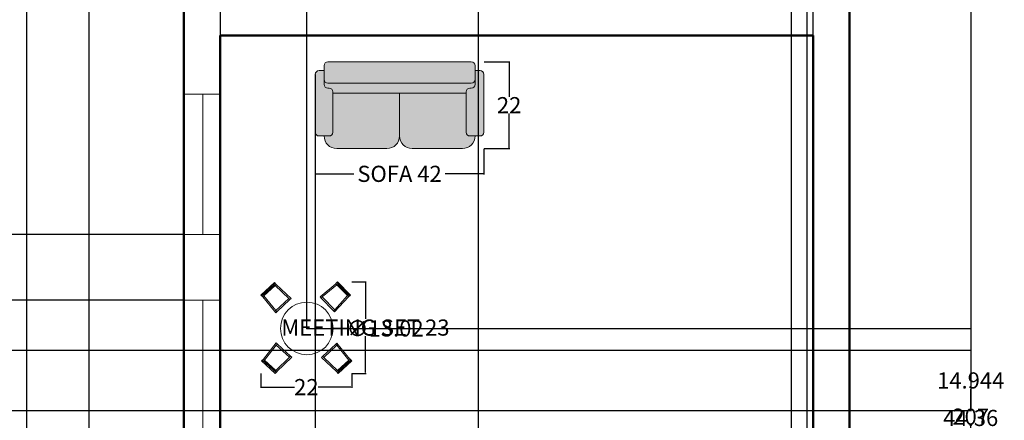
# Model space of a CAD drawing. Units: inches. Extents: x 1454 to 2136, y 626 to 1213.
# Tile 22 of 23: x 1887 to 2131, y 806 to 905. Entities that reach past the tile are written whole.
import ezdxf

# ---------------------------------------------------------------- set-up
doc = ezdxf.new("R2010")
doc.units = ezdxf.units.IN
doc.header["$MEASUREMENT"] = 0
for name, color, linetype, lineweight in [('A-ANNO-DIMS', 2, 'Continuous', 18), ('A-FURN-PATT', 252, 'Continuous', 13), ('A-GLAZ', 4, 'Continuous', 18), ('A-WALL', 7, 'Continuous', 50), ('conference', 41, 'Continuous', 18), ('sofa', 4, 'Continuous', 18)]:
    doc.layers.add(name, color=color, linetype=linetype, lineweight=lineweight)
doc.styles.get("Standard").update_dxf_attribs({"font": 'arial.ttf'})
doc.dimstyles.get("Standard").update_dxf_attribs({"dimtxt": 4, "dimasz": 0.18, "dimexe": 0.18, "dimexo": 0.0625, "dimgap": 0.09, "dimtad": 0, "dimtih": 1, "dimtoh": 1, "dimdec": 0, "dimrnd": 6, "dimzin": 0, "dimdsep": 46, "dimlunit": 3, "dimtxsty": 'Standard', "dimcen": 0.09, "dimadec": 0, "dimazin": 0, "dimtfac": 1, "dimtdec": 0, "dimtofl": 0, "dimtmove": 0, "dimatfit": 3, "dimfxl": 1, "dimtolj": 1, "dimtzin": 0, "dimarcsym": 0})

# ---------------------------------------------------------------- blocks, each defined once
blk = doc.blocks.new('A$C02A636C4')
for p, q in [((0.0679, 0.6401), (0.0679, 0.6013)), ((1.2026, 0.6692), (0.097, 0.6692)), ((1.2317, 0.6401), (1.2317, 0.6013)), ((0, 0.5722), (0, 0.1261)), ((0.0679, 0.6013), (0.0291, 0.6013)), ((0.0679, 0.5334), (0.0679, 0.6013)), ((0.0679, 0.4946), (0.0679, 0.5431)), ((1.2317, 0.6013), (1.2705, 0.6013)), ((1.2317, 0.5334), (1.2317, 0.6013)), ((1.2317, 0.4946), (1.2317, 0.5431)), ((1.2996, 0.5722), (1.2996, 0.1261)), ((1.2026, 0.5043), (0.097, 0.5043)), ((0.1067, 0.4655), (0.097, 0.4655)), ((1.1929, 0.4655), (1.2026, 0.4655)), ((0.1358, 0.1261), (0.1358, 0.4364)), ((1.1638, 0.4267), (0.1358, 0.4267)), ((0.6498, 0.097), (0.6498, 0.4267)), ((1.1638, 0.1261), (1.1638, 0.4364)), ((0.0291, 0.097), (0.1067, 0.097)), ((1.2705, 0.097), (1.1929, 0.097)), ((0.1649, 0), (0.5528, 0)), ((0.7468, 0), (1.1347, 0))]:
    blk.add_line(p, q)
for centre, radius, start, end in [((0.097, 0.6401), 0.0291, 90, 180), ((1.2026, 0.6401), 0.0291, 0, 90), ((0.0291, 0.5722), 0.0291, 90, 180), ((0.097, 0.5334), 0.0291, 180, 270), ((1.2026, 0.5334), 0.0291, 270, 0), ((1.2705, 0.5722), 0.0291, 0, 90), ((0.097, 0.4946), 0.0291, 180, 270), ((0.1067, 0.4364), 0.0291, 0, 90), ((1.1929, 0.4364), 0.0291, 90, 180), ((1.2026, 0.4946), 0.0291, 270, 0), ((0.0291, 0.1261), 0.0291, 180, 270), ((0.1649, 0.097), 0.097, 180, 270), ((0.1067, 0.1261), 0.0291, 270, 0), ((0.5528, 0.097), 0.097, 270, 0), ((0.7468, 0.097), 0.097, 180, 270), ((1.1347, 0.097), 0.097, 270, 0), ((1.1929, 0.1261), 0.0291, 180, 270), ((1.2705, 0.1261), 0.0291, 270, 0)]:
    blk.add_arc(centre, radius, start, end)
blk = doc.blocks.new('ОГ018 на4персон столR500')
for p, q in [((-616, 874), (-872, 635)), ((-601, 858), (-857, 620)), ((-604, 817), (-816, 620)), ((-699, 740), (-713, 755)), ((-705, 761), (-691, 747)), ((-666, 787), (-700, 756)), ((-658, 778), (-672, 793)), ((-664, 800), (-651, 785)), ((-625, 825), (-659, 794)), ((-651, 785), (-658, 778)), ((-612, 811), (-631, 831)), ((-582, 838), (-616, 874)), ((-582, 838), (-604, 817)), ((-340, 571), (-604, 817)), ((-298, 570), (-584, 837)), ((252, 600), (551, 852)), ((294, 600), (571, 832)), ((550, 854), (585, 888)), ((550, 854), (571, 832)), ((570, 873), (813, 621)), ((571, 832), (772, 624)), ((578, 825), (598, 844)), ((585, 888), (829, 636)), ((592, 839), (624, 806)), ((630, 811), (615, 797)), ((615, 797), (622, 790)), ((622, 790), (637, 804)), ((631, 798), (663, 765)), ((669, 771), (654, 757)), ((654, 757), (661, 750)), ((661, 750), (676, 764)), ((670, 758), (702, 725)), ((-838, 599), (-872, 635)), ((-816, 620), (-838, 599)), ((-837, 600), (-591, 297)), ((-809, 626), (-828, 647)), ((-789, 672), (-823, 641)), ((-816, 620), (-589, 339)), ((-781, 663), (-794, 678)), ((-787, 685), (-773, 670)), ((-748, 711), (-782, 679)), ((-773, 670), (-781, 663)), ((-740, 702), (-754, 716)), ((-746, 723), (-732, 708)), ((-707, 749), (-741, 717)), ((-732, 708), (-740, 702)), ((-691, 747), (-699, 740)), ((-589, 339), (-340, 571)), ((-341, 571), (-320, 549)), ((-340, 571), (-320, 549)), ((-320, 549), (-298, 570)), ((-320, 549), (-298, 570)), ((273, 579), (252, 601)), ((273, 579), (252, 600)), ((294, 600), (273, 579)), ((295, 600), (273, 579)), ((509, 334), (273, 579)), ((531, 355), (294, 600)), ((792, 603), (530, 313)), ((772, 624), (531, 355)), ((707, 731), (693, 717)), ((693, 717), (700, 709)), ((700, 709), (714, 723)), ((709, 718), (741, 685)), ((746, 690), (732, 676)), ((732, 676), (739, 669)), ((739, 669), (753, 683)), ((748, 678), (780, 645)), ((765, 631), (785, 650)), ((772, 624), (793, 602)), ((793, 602), (829, 636)), ((-569, 317), (-320, 549)), ((-591, 297), (-569, 317)), ((-591, 297), (-569, 317)), ((-569, 317), (-589, 339)), ((509, 334), (531, 355)), ((530, 313), (509, 334)), ((530, 313), (509, 334)), ((-824, -584), (-582, -277)), ((-803, -603), (-580, -320)), ((-582, -277), (-559, -297)), ((-582, -277), (-559, -297)), ((-559, -297), (-580, -320)), ((-580, -320), (-328, -548)), ((-559, -297), (-308, -526)), ((551, -299), (303, -530)), ((572, -321), (323, -552)), ((573, -278), (551, -299)), ((573, -278), (551, -299)), ((551, -299), (572, -321)), ((799, -601), (572, -321)), ((820, -582), (573, -278)), ((-328, -548), (-588, -798)), ((-285, -546), (-567, -817)), ((-328, -548), (-308, -526)), ((-328, -548), (-308, -526)), ((-308, -526), (-285, -546)), ((-308, -526), (-285, -546)), ((303, -530), (281, -551)), ((303, -530), (281, -551)), ((281, -551), (566, -818)), ((323, -552), (303, -530)), ((323, -552), (303, -530)), ((323, -552), (587, -799)), ((-825, -583), (-859, -619)), ((-599, -855), (-859, -619)), ((-585, -839), (-844, -603)), ((-803, -603), (-825, -583)), ((-796, -610), (-814, -630)), ((-775, -655), (-809, -624)), ((-588, -798), (-803, -603)), ((-767, -646), (-780, -661)), ((-773, -668), (-759, -653)), ((-734, -693), (-768, -662)), ((-759, -653), (-767, -646)), ((-725, -684), (-739, -699)), ((-732, -706), (-718, -691)), ((-692, -731), (-726, -700)), ((-718, -691), (-725, -684)), ((-684, -722), (-697, -736)), ((-690, -743), (-677, -728)), ((-651, -768), (-685, -737)), ((-677, -728), (-684, -722)), ((584, -839), (840, -601)), ((587, -799), (799, -601)), ((599, -855), (855, -617)), ((649, -768), (682, -737)), ((674, -728), (681, -721)), ((688, -743), (674, -728)), ((681, -721), (695, -736)), ((690, -730), (723, -699)), ((715, -690), (722, -683)), ((729, -704), (715, -690)), ((722, -683), (736, -698)), ((731, -692), (764, -661)), ((756, -652), (763, -645)), ((770, -666), (756, -652)), ((763, -645), (777, -659)), ((772, -654), (805, -622)), ((792, -608), (811, -628)), ((799, -601), (821, -580)), ((821, -580), (855, -617)), ((-642, -759), (-656, -774)), ((-649, -781), (-635, -766)), ((-609, -806), (-643, -775)), ((-635, -766), (-642, -759)), ((-596, -791), (-615, -812)), ((-566, -818), (-599, -855)), ((-566, -818), (-588, -798)), ((565, -819), (587, -799)), ((565, -819), (599, -855)), ((594, -792), (613, -812)), ((608, -806), (641, -775)), ((633, -766), (640, -759)), ((647, -781), (633, -766)), ((640, -759), (654, -774))]:
    blk.add_line(p, q)
blk.add_circle((0, 0), 500)
for p in [(-589, 339), (531, 355), (-580, -320), (572, -321)]:
    blk.add_point(p)
blk = doc.blocks.new('WIN-34_84')
blk.add_line((34.84, 4.31), (0, 4.31))
blk.add_lwpolyline([(34.84, 0), (0, 0), (0, 9), (34.84, 9)], close=True)
blk = doc.blocks.new('*D21')
at = {"layer": 'A-ANNO-DIMS', "color": 0, "lineweight": -2, "transparency": 16777216}
for p, q in [((1960.15, 873.16), (1960.15, 866.78)), ((2001.92, 873.16), (2001.92, 866.78)), ((1960.33, 866.96), (1969.73, 866.96)), ((2001.74, 866.96), (1992.34, 866.96))]:
    blk.add_line(p, q, dxfattribs=at)
at = {"layer": 'A-ANNO-DIMS', "color": 0, "transparency": 16777216}
for points in [[(1960.33, 866.99), (1960.33, 866.93), (1960.15, 866.96)], [(2001.74, 866.99), (2001.74, 866.93), (2001.92, 866.96)]]:
    blk.add_solid(points, dxfattribs=at)
at = {"layer": 'Defpoints', "color": 0, "transparency": 16777216}
for p in [(1960.15, 873.22), (2001.92, 873.22), (2001.92, 866.96)]:
    blk.add_point(p, dxfattribs=at)
at = {"layer": 'A-ANNO-DIMS', "color": 0, "transparency": 16777216, "insert": (1981.03, 866.96), "char_height": 4, "attachment_point": 5}
blk.add_mtext('\\A1;SOFA 42', dxfattribs=at)
blk = doc.blocks.new('*D22')
at = {"layer": 'A-ANNO-DIMS', "color": 0, "lineweight": -2, "transparency": 16777216}
for p, q in [((2001.98, 894.73), (2008.36, 894.73)), ((2008.18, 894.55), (2008.18, 886.08)), ((2008.18, 873.4), (2008.18, 881.88)), ((2001.98, 873.22), (2008.36, 873.22))]:
    blk.add_line(p, q, dxfattribs=at)
at = {"layer": 'A-ANNO-DIMS', "color": 0, "transparency": 16777216}
for points in [[(2008.15, 894.55), (2008.21, 894.55), (2008.18, 894.73)], [(2008.15, 873.4), (2008.21, 873.4), (2008.18, 873.22)]]:
    blk.add_solid(points, dxfattribs=at)
at = {"layer": 'Defpoints', "color": 0, "transparency": 16777216}
for p in [(2001.92, 894.73), (2008.18, 894.73), (2001.92, 873.22)]:
    blk.add_point(p, dxfattribs=at)
at = {"layer": 'A-ANNO-DIMS', "color": 0, "transparency": 16777216, "insert": (2008.18, 883.98), "char_height": 4, "attachment_point": 5}
blk.add_mtext('\\A1;22', dxfattribs=at)
blk = doc.blocks.new('*D25')
at = {"layer": 'A-ANNO-DIMS', "color": 0, "lineweight": -2, "transparency": 16777216}
for p, q in [((1969.23, 840.21), (1972.76, 840.21)), ((1972.58, 840.03), (1972.58, 831.02)), ((1972.58, 817.69), (1972.58, 826.7)), ((1969.23, 817.51), (1972.76, 817.51))]:
    blk.add_line(p, q, dxfattribs=at)
at = {"layer": 'A-ANNO-DIMS', "color": 0, "transparency": 16777216}
for points in [[(1972.55, 840.03), (1972.61, 840.03), (1972.58, 840.21)], [(1972.55, 817.69), (1972.61, 817.69), (1972.58, 817.51)]]:
    blk.add_solid(points, dxfattribs=at)
at = {"layer": 'Defpoints', "color": 0, "transparency": 16777216}
for p in [(1969.17, 840.21), (1972.58, 840.21), (1969.17, 817.51)]:
    blk.add_point(p, dxfattribs=at)
at = {"layer": 'A-ANNO-DIMS', "color": 0, "transparency": 16777216, "insert": (1972.58, 828.86), "char_height": 4, "attachment_point": 5}
blk.add_mtext('\\A1;MEETING SET 23', dxfattribs=at)
blk = doc.blocks.new('*D26')
at = {"layer": 'A-ANNO-DIMS', "color": 0, "lineweight": -2, "transparency": 16777216}
for p, q in [((1946.69, 817.45), (1946.69, 813.92)), ((1969.17, 817.45), (1969.17, 813.92)), ((1946.87, 814.1), (1954.96, 814.1)), ((1968.99, 814.1), (1960.9, 814.1))]:
    blk.add_line(p, q, dxfattribs=at)
at = {"layer": 'A-ANNO-DIMS', "color": 0, "transparency": 16777216}
for points in [[(1946.87, 814.13), (1946.87, 814.07), (1946.69, 814.1)], [(1968.99, 814.13), (1968.99, 814.07), (1969.17, 814.1)]]:
    blk.add_solid(points, dxfattribs=at)
at = {"layer": 'Defpoints', "color": 0, "transparency": 16777216}
for p in [(1946.69, 817.51), (1969.17, 817.51), (1969.17, 814.1)]:
    blk.add_point(p, dxfattribs=at)
at = {"layer": 'A-ANNO-DIMS', "color": 0, "transparency": 16777216, "insert": (1957.93, 814.1), "char_height": 4, "attachment_point": 5}
blk.add_mtext('\\A1;22', dxfattribs=at)
blk = doc.blocks.new('*D35')
at = {"layer": 'A-ANNO-DIMS', "color": 0, "lineweight": -2, "transparency": 16777216}
for p, q in [((2092.62, 910.28), (2122.74, 910.28)), ((2122.56, 910.1), (2122.56, 808.91)), ((2122.56, 703.46), (2122.56, 804.65)), ((2092.62, 703.28), (2122.74, 703.28))]:
    blk.add_line(p, q, dxfattribs=at)
at = {"layer": 'A-ANNO-DIMS', "color": 0, "transparency": 16777216}
for points in [[(2122.53, 910.1), (2122.59, 910.1), (2122.56, 910.28)], [(2122.53, 703.46), (2122.59, 703.46), (2122.56, 703.28)]]:
    blk.add_solid(points, dxfattribs=at)
at = {"layer": 'Defpoints', "color": 0, "transparency": 16777216}
for p in [(2092.56, 910.28), (2092.56, 703.28), (2122.56, 703.28)]:
    blk.add_point(p, dxfattribs=at)
at = {"layer": 'A-ANNO-DIMS', "color": 0, "transparency": 16777216, "insert": (2122.56, 806.78), "char_height": 4, "attachment_point": 5}
blk.add_mtext('\\A1;207', dxfattribs=at)
blk = doc.blocks.new('*D37')
at = {"layer": 'A-ANNO-DIMS', "color": 0, "lineweight": -2, "transparency": 16777216}
for p, q in [((1774.56, 712.34), (1774.56, 1210.46)), ((1774.74, 1210.28), (1846.74, 1210.28)), ((1927.38, 1210.28), (1855.38, 1210.28)), ((1927.56, 712.34), (1927.56, 1210.46))]:
    blk.add_line(p, q, dxfattribs=at)
at = {"layer": 'A-ANNO-DIMS', "color": 0, "transparency": 16777216}
for points in [[(1774.74, 1210.31), (1774.74, 1210.25), (1774.56, 1210.28)], [(1927.38, 1210.31), (1927.38, 1210.25), (1927.56, 1210.28)]]:
    blk.add_solid(points, dxfattribs=at)
at = {"layer": 'Defpoints', "color": 0, "transparency": 16777216}
for p in [(1927.56, 1210.28), (1774.56, 712.28), (1927.56, 712.28)]:
    blk.add_point(p, dxfattribs=at)
at = {"layer": 'A-ANNO-DIMS', "color": 0, "transparency": 16777216, "insert": (1851.06, 1210.28), "char_height": 4, "attachment_point": 5}
blk.add_mtext('\\A1;153', dxfattribs=at)
blk = doc.blocks.new('*D53')
at = {"layer": 'A-ANNO-DIMS', "color": 0, "lineweight": -2, "transparency": 16777216}
for p, q in [((1927.57, 851.9), (1462.37, 851.9)), ((1462.55, 851.72), (1462.55, 845.89)), ((1462.55, 835.79), (1462.55, 841.63)), ((1927.57, 835.61), (1462.37, 835.61))]:
    blk.add_line(p, q, dxfattribs=at)
at = {"layer": 'A-ANNO-DIMS', "color": 0, "transparency": 16777216}
for points in [[(1462.52, 851.72), (1462.58, 851.72), (1462.55, 851.9)], [(1462.52, 835.79), (1462.58, 835.79), (1462.55, 835.61)]]:
    blk.add_solid(points, dxfattribs=at)
at = {"layer": 'Defpoints', "color": 0, "transparency": 16777216}
for p in [(1462.55, 851.9), (1927.64, 851.9), (1927.64, 835.61)]:
    blk.add_point(p, dxfattribs=at)
at = {"layer": 'A-ANNO-DIMS', "color": 0, "transparency": 16777216, "insert": (1462.55, 843.76), "char_height": 4, "attachment_point": 5}
blk.add_mtext('\\A1;16.29', dxfattribs=at)
blk = doc.blocks.new('*D57')
at = {"layer": 'A-ANNO-DIMS', "color": 0, "lineweight": -2, "transparency": 16777216}
for p, q in [((1654.43, 823.23), (2122.74, 823.23)), ((2122.56, 823.05), (2122.56, 817.89)), ((2122.56, 808.46), (2122.56, 813.62)), ((1654.62, 808.28), (2122.74, 808.28))]:
    blk.add_line(p, q, dxfattribs=at)
at = {"layer": 'A-ANNO-DIMS', "color": 0, "transparency": 16777216}
for points in [[(2122.53, 823.05), (2122.59, 823.05), (2122.56, 823.23)], [(2122.53, 808.46), (2122.59, 808.46), (2122.56, 808.28)]]:
    blk.add_solid(points, dxfattribs=at)
at = {"layer": 'Defpoints', "color": 0, "transparency": 16777216}
for p in [(1654.37, 823.23), (2122.56, 823.23), (1654.56, 808.28)]:
    blk.add_point(p, dxfattribs=at)
at = {"layer": 'A-ANNO-DIMS', "color": 0, "transparency": 16777216, "insert": (2122.56, 815.75), "char_height": 4, "attachment_point": 5}
blk.add_mtext('\\A1;14.944', dxfattribs=at)
blk = doc.blocks.new('*D61')
at = {"layer": 'A-ANNO-DIMS', "color": 0, "lineweight": -2, "transparency": 16777216}
for p, q in [((1888.56, 1126.22), (1888.56, 628.1)), ((1904.06, 1126.38), (1904.06, 628.1)), ((1888.74, 628.28), (1903.88, 628.28)), ((1904.06, 628.28), (1904.24, 628.28))]:
    blk.add_line(p, q, dxfattribs=at)
at = {"layer": 'A-ANNO-DIMS', "color": 0, "transparency": 16777216}
for points in [[(1888.74, 628.31), (1888.74, 628.25), (1888.56, 628.28)], [(1903.88, 628.31), (1903.88, 628.25), (1904.06, 628.28)]]:
    blk.add_solid(points, dxfattribs=at)
at = {"layer": 'Defpoints', "color": 0, "transparency": 16777216}
for p in [(1888.56, 1126.28), (1904.06, 1126.44), (1904.06, 628.28)]:
    blk.add_point(p, dxfattribs=at)
at = {"layer": 'A-ANNO-DIMS', "color": 0, "transparency": 16777216, "insert": (1912.45, 628.28), "char_height": 4, "attachment_point": 5}
blk.add_mtext('\\A1;15.506', dxfattribs=at)
blk = doc.blocks.new('*D63')
at = {"layer": 'A-ANNO-DIMS', "color": 0, "lineweight": -2, "transparency": 16777216}
for p, q in [((2000.63, 733.98), (2000.63, 1210.46)), ((2000.81, 1210.28), (2034.88, 1210.28)), ((2081.86, 1210.28), (2047.79, 1210.28)), ((2082.04, 733.98), (2082.04, 1210.46))]:
    blk.add_line(p, q, dxfattribs=at)
at = {"layer": 'A-ANNO-DIMS', "color": 0, "transparency": 16777216}
for points in [[(2000.81, 1210.31), (2000.81, 1210.25), (2000.63, 1210.28)], [(2081.86, 1210.31), (2081.86, 1210.25), (2082.04, 1210.28)]]:
    blk.add_solid(points, dxfattribs=at)
at = {"layer": 'Defpoints', "color": 0, "transparency": 16777216}
for p in [(2082.04, 1210.28), (2000.63, 733.92), (2082.04, 733.92)]:
    blk.add_point(p, dxfattribs=at)
at = {"layer": 'A-ANNO-DIMS', "color": 0, "transparency": 16777216, "insert": (2041.33, 1210.28), "char_height": 4, "attachment_point": 5}
blk.add_mtext('\\A1;81.41', dxfattribs=at)
blk = doc.blocks.new('*D83')
at = {"layer": 'A-ANNO-DIMS', "color": 0, "lineweight": -2, "transparency": 16777216}
for p, q in [((1936.64, 835.68), (1936.64, 1210.46)), ((1936.82, 1210.28), (1938.91, 1210.28)), ((1957.86, 1210.28), (1955.77, 1210.28)), ((1958.04, 828.71), (1958.04, 1210.46))]:
    blk.add_line(p, q, dxfattribs=at)
at = {"layer": 'A-ANNO-DIMS', "color": 0, "transparency": 16777216}
for points in [[(1936.82, 1210.31), (1936.82, 1210.25), (1936.64, 1210.28)], [(1957.86, 1210.31), (1957.86, 1210.25), (1958.04, 1210.28)]]:
    blk.add_solid(points, dxfattribs=at)
at = {"layer": 'Defpoints', "color": 0, "transparency": 16777216}
for p in [(1958.04, 1210.28), (1936.64, 835.61), (1958.04, 828.64)]:
    blk.add_point(p, dxfattribs=at)
at = {"layer": 'A-ANNO-DIMS', "color": 0, "transparency": 16777216, "insert": (1947.34, 1210.28), "char_height": 4, "attachment_point": 5}
blk.add_mtext('\\A1;21.407', dxfattribs=at)
blk = doc.blocks.new('*D84')
at = {"layer": 'A-ANNO-DIMS', "color": 0, "lineweight": -2, "transparency": 16777216}
for p, q in [((1958.1, 828.64), (2122.74, 828.64)), ((2122.56, 828.46), (2122.56, 808.6)), ((2122.56, 784.46), (2122.56, 804.33)), ((1936.62, 784.28), (2122.74, 784.28))]:
    blk.add_line(p, q, dxfattribs=at)
at = {"layer": 'A-ANNO-DIMS', "color": 0, "transparency": 16777216}
for points in [[(2122.53, 828.46), (2122.59, 828.46), (2122.56, 828.64)], [(2122.53, 784.46), (2122.59, 784.46), (2122.56, 784.28)]]:
    blk.add_solid(points, dxfattribs=at)
at = {"layer": 'Defpoints', "color": 0, "transparency": 16777216}
for p in [(1958.04, 828.64), (2122.56, 828.64), (1936.56, 784.28)]:
    blk.add_point(p, dxfattribs=at)
at = {"layer": 'A-ANNO-DIMS', "color": 0, "transparency": 16777216, "insert": (2122.56, 806.46), "char_height": 4, "attachment_point": 5}
blk.add_mtext('\\A1;44.36', dxfattribs=at)
blk = doc.blocks.new('*D85')
at = {"layer": 'A-ANNO-DIMS', "color": 0, "lineweight": -2, "transparency": 16777216}
for p, q in [((1936.56, 901.22), (1936.56, 628.1)), ((1960.15, 891.55), (1960.15, 628.1)), ((1936.74, 628.28), (1939.93, 628.28)), ((1959.97, 628.28), (1956.77, 628.28))]:
    blk.add_line(p, q, dxfattribs=at)
at = {"layer": 'A-ANNO-DIMS', "color": 0, "transparency": 16777216}
for points in [[(1936.74, 628.31), (1936.74, 628.25), (1936.56, 628.28)], [(1959.97, 628.31), (1959.97, 628.25), (1960.15, 628.28)]]:
    blk.add_solid(points, dxfattribs=at)
at = {"layer": 'Defpoints', "color": 0, "transparency": 16777216}
for p in [(1936.56, 901.28), (1960.15, 891.61), (1960.15, 628.28)]:
    blk.add_point(p, dxfattribs=at)
at = {"layer": 'A-ANNO-DIMS', "color": 0, "transparency": 16777216, "insert": (1948.35, 628.28), "char_height": 4, "attachment_point": 5}
blk.add_mtext('\\A1;23.594', dxfattribs=at)
blk = doc.blocks.new('*D86')
at = {"layer": 'A-ANNO-DIMS', "color": 0, "lineweight": -2, "transparency": 16777216}
for p, q in [((2078.14, 1210.28), (2077.96, 1210.28)), ((2078.14, 776.98), (2078.14, 1210.46)), ((2083.38, 1210.28), (2078.32, 1210.28)), ((2083.56, 712.34), (2083.56, 1210.46))]:
    blk.add_line(p, q, dxfattribs=at)
at = {"layer": 'A-ANNO-DIMS', "color": 0, "transparency": 16777216}
for points in [[(2078.32, 1210.31), (2078.32, 1210.25), (2078.14, 1210.28)], [(2083.38, 1210.31), (2083.38, 1210.25), (2083.56, 1210.28)]]:
    blk.add_solid(points, dxfattribs=at)
at = {"layer": 'Defpoints', "color": 0, "transparency": 16777216}
for p in [(2078.14, 1210.28), (2078.14, 776.92), (2083.56, 712.28)]:
    blk.add_point(p, dxfattribs=at)
at = {"layer": 'A-ANNO-DIMS', "color": 0, "transparency": 16777216, "insert": (2072.69, 1210.28), "char_height": 4, "attachment_point": 5}
blk.add_mtext('\\A1;5.42', dxfattribs=at)
blk = doc.blocks.new('*D104')
at = {"layer": 'A-ANNO-DIMS', "color": 0, "lineweight": -2, "transparency": 16777216}
for p, q in [((1957.95, 828.64), (1958.13, 828.64)), ((1958.04, 828.55), (1958.04, 828.73)), ((1968.46, 828.64), (1964.73, 828.64))]:
    blk.add_line(p, q, dxfattribs=at)
at = {"layer": 'A-ANNO-DIMS', "color": 0, "transparency": 16777216}
blk.add_solid([(1964.73, 828.67), (1964.73, 828.61), (1964.55, 828.64)], dxfattribs=at)
at = {"layer": 'Defpoints', "color": 0, "transparency": 16777216}
for p in [(1951.53, 828.64), (1964.55, 828.64)]:
    blk.add_point(p, dxfattribs=at)
at = {"layer": 'A-ANNO-DIMS', "color": 0, "transparency": 16777216, "insert": (1977.45, 828.64), "char_height": 4, "attachment_point": 5}
blk.add_mtext('\\A1;∅13.02', dxfattribs=at)

msp = doc.modelspace()

# ---------------------------------------------------------------- hatches: boundary and pattern name
at = {"layer": 'A-FURN-PATT'}
h = msp.add_hatch(dxfattribs=at)
h.set_pattern_fill('ESCHER', color=256)
h.paths.add_polyline_path([(1511.3761, 923.7174, 1), (1525.379, 923.7174, 1)])
h.paths.add_polyline_path([(1525.379, 816.0542, 1), (1511.3761, 816.0542, 1)])
h.paths.add_polyline_path([(1525.379, 712.7345, 1), (1511.3761, 712.7345, 1)])
h.paths.add_polyline_path([(2070.5057, 794.3402, 1), (2056.5027, 794.3402, 1)])
h.paths.add_polyline_path([(2005.868, 1014.5578, 1), (1991.8651, 1014.5578, 1)])
h.paths.add_polyline_path([(1994.0647, 1066.7584, 1), (2008.0677, 1066.7584, 1)])
h.paths.add_polyline_path([(1919.5492, 1065.3848, 1), (1933.5521, 1065.3848, 1)])
h.paths.add_polyline_path([(1936.8517, 1013.7336, 1), (1922.8488, 1013.7336, 1)])
h.paths.add_polyline_path([(1824.6062, 1109.1557, 1), (1838.6091, 1109.1557, 1)])
h = msp.add_hatch(color=256, dxfattribs=at)
h.dxf.hatch_style = 1
h.paths.add_polyline_path([(1855.0231, 1089.5248, 0.41421356), (1850.0231, 1094.5248), (1811.2288, 1094.5248, 0.41421356), (1806.2288, 1089.5248), (1806.2288, 1083.6305, 0.41421356), (1811.2288, 1078.6305), (1850.0231, 1078.6305, 0.41421356), (1855.0231, 1083.6305)])
h.paths.add_polyline_path([(1939.0638, 1089.4209), (1938.9354, 1078.7354, -0.20858653), (1943.5258, 1076.1857), (1952.7682, 1081.5837, 0.24238954)])
h.paths.add_polyline_path([(1939.0638, 1089.4209, 0.00796483), (1938.5148, 1089.4363), (1928.0643, 1089.5619), (1927.936, 1078.8906), (1938.3866, 1078.765, -0.02092855), (1938.9354, 1078.7354)])
h.paths.add_polyline_path([(1928.0643, 1089.5619), (1916.0797, 1089.706), (1916.0698, 1088.8851), (1917.241, 1088.8711, -0.41420041), (1917.7276, 1088.3726), (1917.6308, 1080.3281, -0.41422672), (1917.1324, 1079.8415), (1915.9612, 1079.8556), (1915.9573, 1079.5272, 0.41420799), (1916.4439, 1079.0288), (1927.936, 1078.8906)])
h.paths.add_polyline_path([(1917.7276, 1088.3726, 0.41420041), (1917.241, 1088.8711), (1914.9926, 1088.8981, 0.41421356), (1914.4941, 1088.4115), (1914.3974, 1080.367, 0.41421356), (1914.884, 1079.8686), (1917.1324, 1079.8415, 0.41422672), (1917.6308, 1080.3281)])
h.paths.add_polyline_path([(1928.0939, 1092.0245), (1916.6018, 1092.1627, 0.41422672), (1916.1033, 1091.6761), (1916.0797, 1089.706), (1928.0643, 1089.5619)])
h.paths.add_polyline_path([(1939.0935, 1091.8846, 0.00696804), (1938.5445, 1091.8989), (1928.0939, 1092.0245), (1928.0643, 1089.5619), (1938.5148, 1089.4363, -0.00796483), (1939.0638, 1089.4209)])
h.paths.add_polyline_path([(1939.0935, 1091.8846), (1939.0638, 1089.4209, -0.24238954), (1952.7682, 1081.5837), (1954.897, 1082.827, 0.24500473)])
h.paths.add_polyline_path([(1952.7682, 1081.5837), (1943.5258, 1076.1857, -0.16768112), (1944.8746, 1072.1191), (1944.8073, 1066.5201), (1955.4785, 1066.3918), (1955.5459, 1071.9909, 0.14799784)])
h.paths.add_polyline_path([(1954.897, 1082.827), (1952.7682, 1081.5837, -0.14799784), (1955.5459, 1071.9909), (1955.4785, 1066.3918), (1957.9412, 1066.3622), (1958.0085, 1071.9612, 0.14649407)])
h.paths.add_polyline_path([(1955.4785, 1066.3918), (1944.8073, 1066.5201), (1944.675, 1055.5205, 0.41421356), (1945.1616, 1055.0221), (1945.49, 1055.0181), (1945.5041, 1056.1893, -0.41421356), (1946.0025, 1056.6759), (1954.047, 1056.5792, -0.41421356), (1954.5336, 1056.0807), (1954.5195, 1054.9096), (1955.3404, 1054.8997)])
h.paths.add_polyline_path([(1954.5336, 1056.0807, 0.41421356), (1954.047, 1056.5792), (1946.0025, 1056.6759, 0.41421356), (1945.5041, 1056.1893), (1945.49, 1055.0181), (1945.477, 1053.9409, 0.41422115), (1945.9636, 1053.4425), (1954.0081, 1053.3458, 0.41420598), (1954.5066, 1053.8324)])
h.paths.add_polyline_path([(1957.9412, 1066.3622), (1955.4785, 1066.3918), (1955.3404, 1054.8997), (1957.3105, 1054.876, 0.41421356), (1957.8089, 1055.3626)])
h.paths.add_polyline_path([(1974.6911, 1066.3918), (1972.2285, 1066.3622), (1972.3608, 1055.3626, 0.41421356), (1972.8592, 1054.876), (1974.8293, 1054.8997)])
h.paths.add_polyline_path([(1985.3624, 1066.5201), (1974.6911, 1066.3918), (1974.8293, 1054.8997), (1975.6501, 1054.9096), (1975.6361, 1056.0807, -0.41421356), (1976.1227, 1056.5792), (1984.1672, 1056.6759, -0.41421356), (1984.6656, 1056.1893), (1984.6797, 1055.0181), (1985.008, 1055.0221, 0.41421356), (1985.4946, 1055.5205)])
h.paths.add_polyline_path([(1984.6656, 1056.1893, 0.41421356), (1984.1672, 1056.6759), (1976.1227, 1056.5792, 0.41421356), (1975.6361, 1056.0807), (1975.6631, 1053.8324, 0.41422115), (1976.1615, 1053.3458), (1984.206, 1053.4425, 0.41420597), (1984.6926, 1053.9409)])
h.paths.add_polyline_path([(1985.2951, 1072.1191, -0.16768112), (1986.6438, 1076.1857), (1977.4014, 1081.5837, 0.14799988), (1974.6238, 1071.9907), (1974.6911, 1066.3918), (1985.3624, 1066.5201)])
h.paths.add_polyline_path([(1977.4014, 1081.5837), (1975.2727, 1082.827, 0.14649407), (1972.1612, 1071.9612), (1972.2285, 1066.3622), (1974.6911, 1066.3918), (1974.6238, 1071.9907, -0.14799988)])
h.paths.add_polyline_path([(1991.1058, 1089.4209, 0.24238954), (1977.4014, 1081.5837), (1986.6438, 1076.1857, -0.20858653), (1991.2343, 1078.7354)])
h.paths.add_polyline_path([(1991.1058, 1089.4209), (1991.0762, 1091.8846, 0.24500473), (1975.2727, 1082.827), (1977.4014, 1081.5837, -0.24238954)])
h.paths.add_polyline_path([(2002.1053, 1089.5619), (1991.6547, 1089.4363, 0.00796283), (1991.1058, 1089.4209), (1991.2343, 1078.7354, -0.02092855), (1991.783, 1078.765), (2002.2336, 1078.8906)])
h.paths.add_polyline_path([(2002.0757, 1092.0245), (1991.6251, 1091.8989, 0.00696804), (1991.0762, 1091.8846), (1991.1058, 1089.4209, -0.00796283), (1991.6547, 1089.4363), (2002.1053, 1089.5619)])
h.paths.add_polyline_path([(2014.0663, 1091.6761, 0.4142004), (2013.5679, 1092.1627), (2002.0757, 1092.0245), (2002.1053, 1089.5619), (2014.09, 1089.706)])
h.paths.add_polyline_path([(2012.4421, 1088.3726, -0.41422672), (2012.9287, 1088.8711), (2014.0999, 1088.8851), (2014.09, 1089.706), (2002.1053, 1089.5619), (2002.2336, 1078.8906), (2013.7258, 1079.0288, 0.41421913), (2014.2124, 1079.5273), (2014.2084, 1079.8556), (2013.0373, 1079.8415, -0.4142004), (2012.5388, 1080.3281)])
h.paths.add_polyline_path([(1986.6438, 1024.0964), (1977.4014, 1029.4944, 0.14799988), (1974.6238, 1019.9014), (1974.6911, 1014.3025), (1985.3624, 1014.4308), (1985.2951, 1020.0298, -0.16768112)])
h.paths.add_polyline_path([(1991.1058, 1037.3316, 0.24238954), (1977.4014, 1029.4944), (1986.6438, 1024.0964, -0.20858653), (1991.2343, 1026.6461)])
h.paths.add_polyline_path([(2002.1053, 1037.4726), (1991.6547, 1037.347, 0.00796283), (1991.1058, 1037.3316), (1991.2343, 1026.6461, -0.02092855), (1991.783, 1026.6757), (2002.2336, 1026.8013)])
h.paths.add_polyline_path([(2012.4421, 1036.2833, -0.41422672), (2012.9287, 1036.7818), (2014.0999, 1036.7958), (2014.09, 1037.6167), (2002.1053, 1037.4726), (2002.2336, 1026.8013), (2013.7258, 1026.9395, 0.41421913), (2014.2124, 1027.438), (2014.2084, 1027.7663), (2013.0373, 1027.7522, -0.4142004), (2012.5388, 1028.2388)])
h.paths.add_polyline_path([(2015.6755, 1036.3222, 0.41421356), (2015.1771, 1036.8088), (2012.9287, 1036.7818, 0.41422672), (2012.4421, 1036.2833), (2012.5388, 1028.2388, 0.4142004), (2013.0373, 1027.7522), (2015.2856, 1027.7793, 0.41421356), (2015.7722, 1028.2777)])
h.paths.add_polyline_path([(1985.3624, 1014.4308), (1974.6911, 1014.3025), (1974.8293, 1002.8104), (1975.6501, 1002.8203), (1975.6361, 1003.9914, -0.41421356), (1976.1227, 1004.4899), (1984.1672, 1004.5866, -0.41421356), (1984.6656, 1004.1), (1984.6797, 1002.9288), (1985.008, 1002.9328, 0.41421356), (1985.4946, 1003.4312)])
h.paths.add_polyline_path([(1984.6656, 1004.1, 0.41421356), (1984.1672, 1004.5866), (1976.1227, 1004.4899, 0.41421356), (1975.6361, 1003.9914), (1975.6631, 1001.743, 0.41422115), (1976.1615, 1001.2564), (1984.206, 1001.3532, 0.41420598), (1984.6926, 1001.8516)])
h.paths.add_polyline_path([(1974.6911, 1014.3025), (1972.2285, 1014.2729), (1972.3608, 1003.2733, 0.41421356), (1972.8592, 1002.7867), (1974.8293, 1002.8104)])
h.paths.add_polyline_path([(1974.6238, 1019.9014, -0.14799988), (1977.4014, 1029.4944), (1975.2727, 1030.7376, 0.14649407), (1972.1612, 1019.8719), (1972.2285, 1014.2729), (1974.6911, 1014.3025)])
h.paths.add_polyline_path([(1991.1058, 1037.3316), (1991.0762, 1039.7953, 0.24500473), (1975.2727, 1030.7376), (1977.4014, 1029.4944, -0.24238954)])
h.paths.add_polyline_path([(2002.0757, 1039.9352), (1991.6251, 1039.8096, 0.00696804), (1991.0762, 1039.7953), (1991.1058, 1037.3316, -0.00796283), (1991.6547, 1037.347), (2002.1053, 1037.4726)])
h.paths.add_polyline_path([(2014.0663, 1039.5868, 0.4142004), (2013.5679, 1040.0734), (2002.0757, 1039.9352), (2002.1053, 1037.4726), (2014.09, 1037.6167)])
h.paths.add_polyline_path([(1955.5459, 1019.9016, 0.14799784), (1952.7682, 1029.4944), (1943.5258, 1024.0964, -0.16768112), (1944.8746, 1020.0298), (1944.8073, 1014.4308), (1955.4785, 1014.3025)])
h.paths.add_polyline_path([(1955.4785, 1014.3025), (1944.8073, 1014.4308), (1944.675, 1003.4312, 0.41421356), (1945.1616, 1002.9328), (1945.49, 1002.9288), (1945.5041, 1004.1, -0.41421356), (1946.0025, 1004.5866), (1954.047, 1004.4899, -0.41421356), (1954.5336, 1003.9914), (1954.5195, 1002.8203), (1955.3404, 1002.8104)])
h.paths.add_polyline_path([(1939.0638, 1037.3316), (1938.9354, 1026.6461, -0.20858653), (1943.5258, 1024.0964), (1952.7682, 1029.4944, 0.24238954)])
h.paths.add_polyline_path([(1939.0638, 1037.3316, 0.00796483), (1938.5148, 1037.347), (1928.0643, 1037.4726), (1927.936, 1026.8013), (1938.3866, 1026.6757, -0.02092855), (1938.9354, 1026.6461)])
h.paths.add_polyline_path([(1928.0643, 1037.4726), (1916.0797, 1037.6167), (1916.0698, 1036.7958), (1917.241, 1036.7818, -0.41420041), (1917.7276, 1036.2833), (1917.6308, 1028.2388, -0.41422672), (1917.1324, 1027.7522), (1915.9612, 1027.7663), (1915.9573, 1027.4379, 0.41420799), (1916.4439, 1026.9395), (1927.936, 1026.8013)])
h.paths.add_polyline_path([(1917.7276, 1036.2833, 0.41420041), (1917.241, 1036.7818), (1914.9926, 1036.8088, 0.41421356), (1914.4941, 1036.3222), (1914.3974, 1028.2777, 0.41421356), (1914.884, 1027.7793), (1917.1324, 1027.7522, 0.41422672), (1917.6308, 1028.2388)])
h.paths.add_polyline_path([(1928.0939, 1039.9352), (1916.6018, 1040.0734, 0.41422672), (1916.1033, 1039.5868), (1916.0797, 1037.6167), (1928.0643, 1037.4726)])
h.paths.add_polyline_path([(1939.0935, 1039.7953, 0.00696804), (1938.5445, 1039.8096), (1928.0939, 1039.9352), (1928.0643, 1037.4726), (1938.5148, 1037.347, -0.00796483), (1939.0638, 1037.3316)])
h.paths.add_polyline_path([(1939.0935, 1039.7953), (1939.0638, 1037.3316, -0.24238954), (1952.7682, 1029.4944), (1954.897, 1030.7376, 0.24500473)])
h.paths.add_polyline_path([(1954.897, 1030.7376), (1952.7682, 1029.4944, -0.14799784), (1955.5459, 1019.9016), (1955.4785, 1014.3025), (1957.9412, 1014.2729), (1958.0085, 1019.8719, 0.14649407)])
h.paths.add_polyline_path([(1957.9412, 1014.2729), (1955.4785, 1014.3025), (1955.3404, 1002.8104), (1957.3105, 1002.7867, 0.41421356), (1957.8089, 1003.2733)])
h.paths.add_polyline_path([(1954.5336, 1003.9914, 0.41421356), (1954.047, 1004.4899), (1946.0025, 1004.5866, 0.41421356), (1945.5041, 1004.1), (1945.49, 1002.9288), (1945.477, 1001.8516, 0.41422115), (1945.9636, 1001.3532), (1954.0081, 1001.2564, 0.41420598), (1954.5066, 1001.743)])
h.paths.add_polyline_path([(1997.553, 886.9384), (1981.0334, 886.9384), (1981.0334, 876.3409, 0.41421356), (1984.1503, 873.224), (1996.6179, 873.224, 0.41421356), (1999.7348, 876.3409), (1998.488, 876.3409, -0.41421356), (1997.553, 877.276)])
h.paths.add_polyline_path([(1981.0334, 886.9384), (1964.5139, 886.9384), (1964.5139, 877.276, -0.41421356), (1963.5788, 876.3409), (1962.3321, 876.3409, 0.41421356), (1965.449, 873.224), (1977.9165, 873.224, 0.41421356), (1981.0334, 876.3409)])
h.paths.add_polyline_path([(1964.5139, 886.9384), (1964.5139, 887.25, 0.47353022), (1963.4209, 888.1978, -0.46345458), (1962.3321, 889.1202), (1962.3321, 890.6786), (1962.3321, 892.5488), (1961.0853, 892.5488, 0.41421356), (1960.1503, 891.6137), (1960.1503, 877.276, 0.41421356), (1961.0853, 876.3409), (1963.5788, 876.3409, 0.41421356), (1964.5139, 877.276)])
h.paths.add_polyline_path([(1999.7348, 892.5488), (1999.7348, 893.7955, 0.41421356), (1998.7997, 894.7306), (1963.2672, 894.7306, 0.41421356), (1962.3321, 893.7955), (1962.3321, 892.5488), (1962.3321, 890.3669, 0.41421356), (1963.2672, 889.4319), (1998.7997, 889.4319, 0.41421356), (1999.7348, 890.3669), (1999.7348, 890.6786)])
h.paths.add_polyline_path([(2001.9166, 891.6137, 0.41421356), (2000.9815, 892.5488), (1999.7348, 892.5488), (1999.7348, 890.6786), (1999.7348, 890.3669), (1999.7348, 889.1202, -0.41421356), (1998.7997, 888.1851), (1998.488, 888.1851, 0.41421356), (1997.553, 887.25), (1997.553, 877.276, 0.41421356), (1998.488, 876.3409), (1999.7348, 876.3409), (2000.9815, 876.3409, 0.41421356), (2001.9166, 877.276)])
h.paths.add_polyline_path([(1999.7348, 889.1202), (1999.7348, 890.3669, -0.41421356), (1998.7997, 889.4319), (1963.2672, 889.4319, -0.41421356), (1962.3321, 890.3669), (1962.3321, 889.1202, 0.46345458), (1963.4209, 888.1978, -0.45647258), (1964.5139, 887.3025), (1964.5139, 886.9384), (1997.553, 886.9384), (1997.553, 887.25, -0.41421356), (1998.488, 888.1851), (1998.7997, 888.1851, 0.41421356)])
h.paths.add_polyline_path([(1540.5701, 966.1379, 0.41421356), (1538.9915, 967.7165), (1523.2061, 967.7165, 0.41421356), (1521.6275, 966.1379), (1521.6275, 964.5679, 0.41579661), (1523.2061, 962.9808), (1538.9915, 962.9808, 0.41421356), (1540.5701, 964.5594)])
h.paths.add_polyline_path([(1538.9151, 960.1995, 0.41421356), (1537.968, 961.1466), (1524.2565, 961.1466, 0.41421356), (1523.3094, 960.1995), (1523.3094, 947.859, 0.41421356), (1524.2565, 946.9119), (1537.968, 946.9119, 0.41421356), (1538.9151, 947.859)])
h.paths.add_polyline_path([(1555.8609, 960.5704, 0.41421356), (1554.9138, 961.5176), (1543.8299, 961.5176, 0.41421356), (1542.8828, 960.5704), (1542.8828, 946.859, 0.41421356), (1543.8299, 945.9119), (1554.9138, 945.9119, 0.41421356), (1555.8609, 946.859)])
h.paths.add_polyline_path([(1555.8609, 941.6364, 0.41421356), (1554.9138, 942.5835), (1543.8299, 942.5835, 0.41421356), (1542.8828, 941.6364), (1542.8828, 927.9249, 0.41421356), (1543.8299, 926.9778), (1554.9138, 926.9778, 0.41421356), (1555.8609, 927.9249)])
h.paths.add_polyline_path([(1555.8609, 922.6938, 0.41421356), (1554.9138, 923.6409), (1543.8299, 923.6409, 0.41421356), (1542.8828, 922.6938), (1542.8828, 908.9824, 0.41421356), (1543.8299, 908.0352), (1554.9138, 908.0352, 0.41421356), (1555.8609, 908.9824)])
h.paths.add_polyline_path([(1555.8609, 815.2921, 0.41421356), (1554.9138, 816.2392), (1543.8299, 816.2392, 0.41421356), (1542.8828, 815.2921), (1542.8828, 801.5806, 0.41421356), (1543.8299, 800.6335), (1554.9138, 800.6335, 0.41421356), (1555.8609, 801.5806)])
h.paths.add_polyline_path([(1555.8609, 834.2346, 0.41421356), (1554.9138, 835.1818), (1543.8299, 835.1818, 0.41421356), (1542.8828, 834.2346), (1542.8828, 820.5232, 0.41421356), (1543.8299, 819.576), (1554.9138, 819.576, 0.41421356), (1555.8609, 820.5232)])
h.paths.add_polyline_path([(1555.8609, 853.1687, 0.41421356), (1554.9138, 854.1158), (1543.8299, 854.1158, 0.41421356), (1542.8828, 853.1687), (1542.8828, 839.4572, 0.41421356), (1543.8299, 838.5101), (1554.9138, 838.5101, 0.41421356), (1555.8609, 839.4572)])
h.paths.add_polyline_path([(1538.9151, 852.7977, 0.41421356), (1537.968, 853.7448), (1524.2565, 853.7448, 0.41421356), (1523.3094, 852.7977), (1523.3094, 840.4573, 0.41421356), (1524.2565, 839.5101), (1537.968, 839.5101, 0.41421356), (1538.9151, 840.4573)])
h.paths.add_polyline_path([(1538.9151, 748.5053, 0.41421356), (1537.968, 749.4524), (1524.2565, 749.4524, 0.41421356), (1523.3094, 748.5053), (1523.3094, 736.1648, 0.41421356), (1524.2565, 735.2177), (1537.968, 735.2177, 0.41421356), (1538.9151, 736.1648)])
h.paths.add_polyline_path([(1555.8609, 748.8763, 0.41421356), (1554.9138, 749.8234), (1543.8299, 749.8234, 0.41421356), (1542.8828, 748.8763), (1542.8828, 735.1648, 0.41421356), (1543.8299, 734.2177), (1554.9138, 734.2177, 0.41421356), (1555.8609, 735.1648)])
h.paths.add_polyline_path([(1555.8609, 729.9422, 0.41421356), (1554.9138, 730.8893), (1543.8299, 730.8893, 0.41421356), (1542.8828, 729.9422), (1542.8828, 716.2308, 0.41421356), (1543.8299, 715.2836), (1554.9138, 715.2836, 0.41421356), (1555.8609, 716.2308)])
h.paths.add_polyline_path([(1555.8609, 710.9996, 0.41421356), (1554.9138, 711.9468), (1543.8299, 711.9468, 0.41421356), (1542.8828, 710.9996), (1542.8828, 697.2882, 0.41421356), (1543.8299, 696.3411), (1554.9138, 696.3411, 0.41421356), (1555.8609, 697.2882)])
h.paths.add_polyline_path([(1562.4308, 712.0232, 0.44500955), (1560.6884, 713.5932), (1559.1098, 713.5932, 0.3840739), (1557.6951, 712.0232), (1557.6951, 696.2377, 0.43158582), (1559.3667, 694.6619), (1560.9452, 694.6619, 0.39705211), (1562.4308, 696.2377)])
h.paths.add_polyline_path([(1559.2737, 713.6017, -0.41421356), (1557.6951, 715.1803), (1557.6951, 730.9658, -0.39284205), (1559.1577, 732.5401, -0.39284205), (1557.6951, 734.1143), (1557.6951, 749.8998, -0.41421356), (1559.2737, 751.4784), (1560.8522, 751.4784, -0.41421356), (1562.4308, 749.8998), (1562.4308, 734.1143, -0.39284205), (1560.9682, 732.5401, -0.39284205), (1562.4308, 730.9658), (1562.4308, 715.1803, -0.41421356), (1560.8522, 713.6017), (1559.2737, 713.5932), (1559.4375, 713.5932, 0.05204098), (1559.1098, 713.5932)])
h.paths.add_polyline_path([(1559.2737, 732.5443), (1559.2737, 732.5358), (1560.8522, 732.5358), (1560.8522, 732.5443)], flags=16)
h.paths.add_polyline_path([(1562.4308, 749.8998, 0.41421356), (1560.8522, 751.4784), (1559.2737, 751.4784, 0.41421356), (1557.6951, 749.8998), (1557.6951, 734.1143, 0.41421356), (1559.2737, 732.5358), (1559.2737, 732.5443, 0.41421356), (1557.6951, 730.9658), (1557.6951, 715.1803, 0.41421356), (1559.2737, 713.6017), (1560.8437, 713.6018, 0.41579661), (1562.4308, 715.1803), (1562.4308, 730.9658, 0.41421356), (1560.8522, 732.5443), (1560.8522, 732.5358, 0.41421356), (1562.4308, 734.1143)])

# ---------------------------------------------------------------- linework, layer by layer
at = {"layer": 'A-WALL'}
for p, q in [((1927.5563, 784.2825), (1927.5563, 910.2825)), ((2092.5563, 703.2825), (2092.5563, 910.2825)), ((2083.5563, 901.2825), (1936.5563, 901.2825)), ((1936.5563, 784.2825), (1936.5563, 901.2825)), ((2083.5563, 712.2825), (2083.5563, 901.2825))]:
    msp.add_line(p, q, dxfattribs=at)

# ---------------------------------------------------------------- block references
at = {"layer": 'A-GLAZ'}
for p, rotation in [((1936.6352, 851.9027), 89.99999999999913), ((1936.6352, 800.7734), 89.9999999999993)]:
    msp.add_blockref('WIN-34_84', p, dxfattribs=dict(at, rotation=rotation))
at = {"layer": 'conference', "xscale": 0.0130203793305502, "yscale": 0.0130203793305502, "zscale": 0.0130203793305502}
msp.add_blockref('ОГ018 на4персон столR500', (1958.0422, 828.6443), dxfattribs=at)
at = {"layer": 'sofa', "xscale": 32.13736766467667, "yscale": 32.13736766467667, "zscale": 32.13736766467667}
msp.add_blockref('A$C02A636C4', (1960.1503, 873.224), dxfattribs=at)

# ---------------------------------------------------------------- dimensions: what is measured, and where the dimension line sits
at = {"layer": 'A-ANNO-DIMS'}
for base, p1, p2, override, picture, middle in [((1927.5563, 1210.2845), (1774.5563, 712.2825), (1927.5563, 712.2825), {"dimdec": 0, "dimlfac": 1, "dimrnd": 0, "dimzin": 0, "dimdsep": 46, "dimlunit": 2}, '*D37', (1851.0563, 1210.2845)), ((1958.0422, 1210.2845), (1936.6352, 835.6136), (1958.0422, 828.6443), {"dimdec": 3, "dimlfac": 1, "dimrnd": 0, "dimzin": 0, "dimdsep": 46, "dimlunit": 2}, '*D83', (1947.3387, 1210.2845)), ((2082.0362, 1210.2845), (2000.6276, 733.9205), (2082.0362, 733.9205), {"dimdec": 2, "dimlfac": 1, "dimrnd": 0, "dimzin": 0, "dimdsep": 46, "dimlunit": 2}, '*D63', (2041.3319, 1210.2845)), ((2078.1364, 1210.2845), (2083.5563, 712.2825), (2078.1364, 776.9179), {"dimdec": 2, "dimlfac": 1, "dimrnd": 0, "dimzin": 0, "dimdsep": 46, "dimlunit": 2}, '*D86', (2072.6917, 1210.2845)), ((1904.0619, 628.2805), (1888.5563, 1126.2825), (1904.0619, 1126.439), {"dimdec": 3, "dimlfac": 1, "dimrnd": 0, "dimzin": 0, "dimdsep": 46, "dimlunit": 2}, '*D61', (1912.4452, 628.2805)), ((1960.1503, 628.2805), (1936.5563, 901.2825), (1960.1503, 891.6137), {"dimdec": 3, "dimlfac": 1, "dimrnd": 0, "dimzin": 0, "dimdsep": 46, "dimlunit": 2}, '*D85', (1948.3533, 628.2805)), ((1969.1706, 814.1032), (1946.6868, 817.5079), (1969.1706, 817.5079), {"dimdec": 0, "dimlfac": 1, "dimrnd": 0, "dimzin": 0, "dimdsep": 46, "dimlunit": 2}, '*D26', (1957.9287, 814.1032))]:
    dim = msp.add_linear_dim(base=base, p1=p1, p2=p2, dimstyle='Standard', override=override, dxfattribs=at)
    dim.commit()
    dim.dimension.update_dxf_attribs({"geometry": picture, "text_midpoint": middle})
for base, p1, p2, override, picture, middle in [((2122.5583, 703.2825), (2092.5563, 910.2825), (2092.5563, 703.2825), {"dimdec": 0, "dimlfac": 1, "dimrnd": 0, "dimzin": 0, "dimdsep": 46, "dimlunit": 2}, '*D35', (2122.5583, 806.7825)), ((2008.1816, 894.7306), (2001.9166, 873.224), (2001.9166, 894.7306), {"dimdec": 0, "dimlfac": 1, "dimrnd": 0, "dimzin": 0, "dimdsep": 46, "dimlunit": 2}, '*D22', (2008.1816, 883.9773)), ((1462.5543, 851.9027), (1927.6352, 835.6136), (1927.6352, 851.9027), {"dimdec": 2, "dimlfac": 1, "dimrnd": 0, "dimzin": 0, "dimdsep": 46, "dimlunit": 2}, '*D53', (1462.5543, 843.7581)), ((2122.5583, 828.6443), (1936.5563, 784.2825), (1958.0422, 828.6443), {"dimdec": 2, "dimlfac": 1, "dimrnd": 0, "dimzin": 0, "dimdsep": 46, "dimlunit": 2}, '*D84', (2122.5583, 806.4634)), ((2122.5583, 823.2266), (1654.5563, 808.2825), (1654.3723, 823.2266), {"dimdec": 3, "dimlfac": 1, "dimrnd": 0, "dimzin": 0, "dimdsep": 46, "dimlunit": 2}, '*D57', (2122.5583, 815.7545))]:
    dim = msp.add_linear_dim(base=base, p1=p1, p2=p2, angle=90, dimstyle='Standard', override=override, dxfattribs=at)
    dim.commit()
    dim.dimension.update_dxf_attribs({"geometry": picture, "text_midpoint": middle})
dim = msp.add_linear_dim(base=(2001.9166, 866.9591), p1=(1960.1503, 873.224), p2=(2001.9166, 873.224), text='SOFA <>', dimstyle='Standard', override={"dimdec": 0, "dimlfac": 1, "dimrnd": 0, "dimzin": 0, "dimdsep": 46, "dimlunit": 2}, dxfattribs=at)
dim.commit()
dim.dimension.update_dxf_attribs({"geometry": '*D21', "text_midpoint": (1981.0334, 866.9591)})
dim = msp.add_linear_dim(base=(1972.5753, 840.2055), p1=(1969.1706, 817.5079), p2=(1969.1706, 840.2055), angle=90, text='MEETING SET <>', dimstyle='Standard', override={"dimdec": 0, "dimlfac": 1, "dimrnd": 0, "dimzin": 0, "dimdsep": 46, "dimlunit": 2}, dxfattribs=at)
dim.commit()
dim.dimension.update_dxf_attribs({"geometry": '*D25', "text_midpoint": (1972.5753, 828.8567)})
dim = msp.add_diameter_dim_2p(p1=(1951.532, 828.6447), p2=(1964.5524, 828.644), dimstyle='Standard', override={"dimdec": 2, "dimlfac": 1, "dimrnd": 0, "dimzin": 0, "dimdsep": 46, "dimlunit": 2}, dxfattribs=at)
dim.commit()
dim.dimension.update_dxf_attribs({"geometry": '*D104', "text_midpoint": (1968.4585, 828.6438), "dimtype": 163})

doc.saveas('drawing.dxf')
